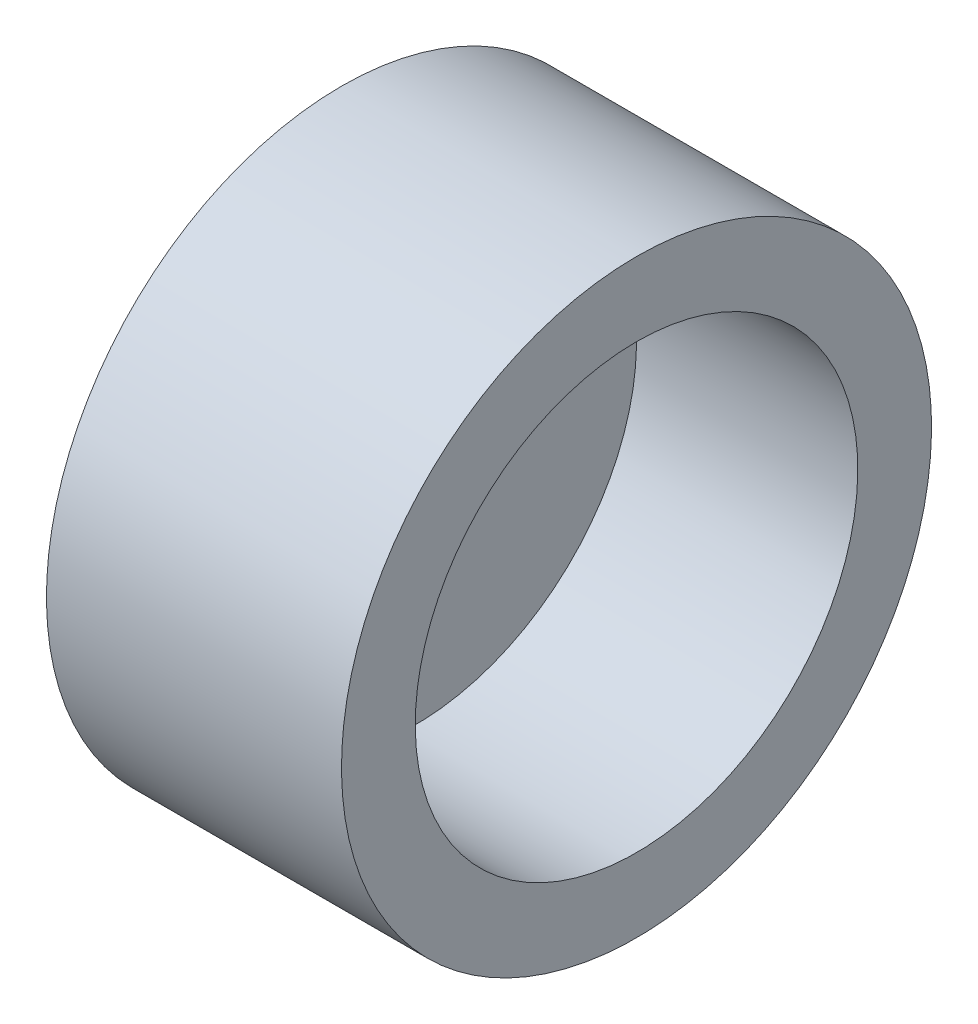
SolidWorks part; units mm, degrees
material "Plain Carbon Steel"
ref_plane "Front Plane" through (0, 0, 0) normal (0, 0, 1) x (1, 0, 0)
ref_plane "Top Plane" through (0, 0, 0) normal (0, 1, 0) x (1, 0, 0)
ref_plane "Right Plane" through (0, 0, 0) normal (1, 0, 0) x (0, 0, -1)
sketch "Cup Profile Sketch" plane through (0, 0, 0) normal (0, 0, 1) x (1, 0, 0)
  line L0 (-19.05, 0) -> (-25.4, 0)
  line L1 (-25.4, 0) -> (-25.4, 25.4)
  line L3 (0, 25.4) -> (0, 19.05)
  line L4 (-25.4, 25.4) -> (0, 25.4)
  line L5 (-19.05, 0) -> (-19.05, 19.05)
  line L6 (-19.05, 19.05) -> (0, 19.05)
  line L7 (0, 0) -> (0, 34.1976) construction
  dimension "D1" = 25.4
  dimension "D2" = 25.4
  dimension "D3" = 19.05
  dimension "D4" = 19.05
revolve "Cup Body Revolve" add sketch "Cup Profile Sketch" angle 360 about L0
hole_wizard "Countersunk Centre Hole" positions "3DSketch1" profile "Sketch4" countersink size "#0" standard "ANSI Inch"
sketch3d "3DSketch1"
  point P0 (0, 0, 0)
  point P3 (-25.4, 0, 0)
sketch "Sketch4" plane through (-25.4, 0, 0) normal (0, 1, 0) x (0, 0, 1)
  line L0 (0, 0) -> (0, 21.1104)
  line L1 (0, 21.1104) -> (3.429, 19.05)
  line L2 (3.429, 19.05) -> (3.429, 3.6524)
  line L3 (3.429, 3.6524) -> (6.604, 0)
  line L5 (6.604, 0) -> (0, 0)
  line L6 (-3.429, 3.6524) -> (-6.604, 0) construction
  line L10 (0, 21.1104) -> (-3.429, 19.05) construction
  line L11 (0, -6.35) -> (0, 107.95) construction
  dimension "Hole Dia." = 6.858
  dimension "Hole Depth" = 19.05
  dimension "Near C'Sink Dia." = 13.208
  dimension "Near C'Sink Angle" = 82
  dimension "Drill Angle" = 118
